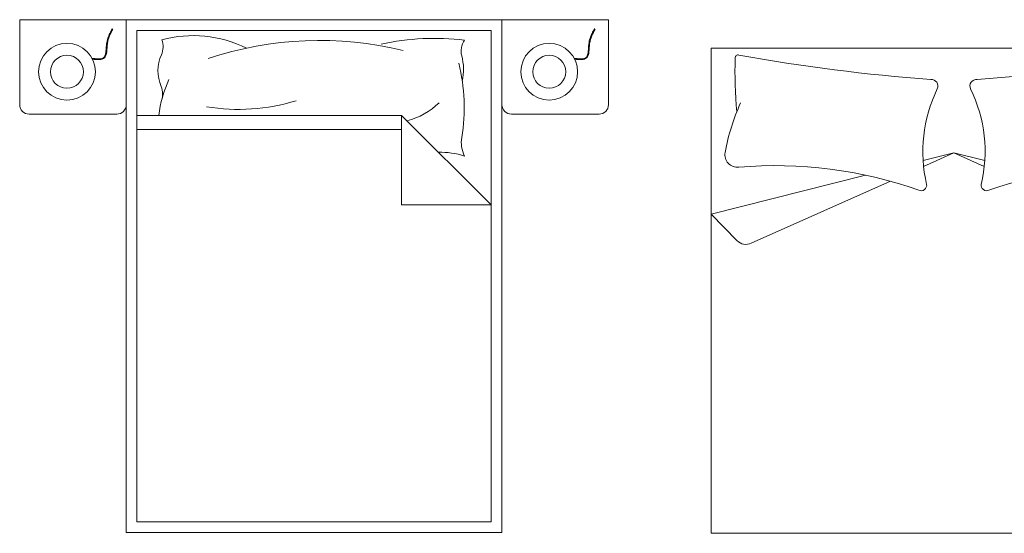
# Model space of a CAD drawing. Units: inches. Extents: x 1994 to 3075, y 3517 to 3950.
# Tile 31 of 58: x 1994.4409 to 1994.6046, y 3553.7994 to 3553.885. Entities that reach past the tile are written whole.
import ezdxf

# ---------------------------------------------------------------- set-up
doc = ezdxf.new("R2010")
doc.units = ezdxf.units.IN
doc.layers.add('A-FURN-REFR', color=8, linetype='Continuous', lineweight=13)

msp = doc.modelspace()

# ---------------------------------------------------------------- linework, layer by layer
at = {"layer": 'A-FURN-REFR'}
for p, q in [((1994.458602013046, 3553.884958485291), (1994.440885477613, 3553.884958485291)), ((1994.440885477613, 3553.884958485291), (1994.440885477613, 3553.870803096903)), ((1994.458602013046, 3553.884958485291), (1994.52109023475, 3553.884958485291)), ((1994.458602013046, 3553.799561227223), (1994.458602013046, 3553.884958485291)), ((1994.458602013046, 3553.870803096903), (1994.458602013046, 3553.884958485291)), ((1994.52109023475, 3553.799561227223), (1994.52109023475, 3553.884958485291)), ((1994.538806770183, 3553.884958485291), (1994.52109023475, 3553.884958485291)), ((1994.52109023475, 3553.884958485291), (1994.52109023475, 3553.870803096903)), ((1994.538806770183, 3553.870803096903), (1994.538806770183, 3553.884958485291)), ((1994.460391562079, 3553.801350776257), (1994.460391562079, 3553.883168936257)), ((1994.460391562079, 3553.883168936257), (1994.519300685716, 3553.883168936257)), ((1994.519300685716, 3553.883168936257), (1994.519300685716, 3553.801350776257)), ((1994.555875329129, 3553.880219755423), (1994.596260242865, 3553.880219755423)), ((1994.555875329129, 3553.880219755423), (1994.596260242865, 3553.880219755423)), ((1994.555875329129, 3553.799449927951), (1994.555875329129, 3553.880219755423)), ((1994.636645156601, 3553.880219755423), (1994.596260242865, 3553.880219755423)), ((1994.636645156601, 3553.880219755423), (1994.596260242865, 3553.880219755423)), ((1994.442460280762, 3553.869228293754), (1994.457027209896, 3553.869228293754)), ((1994.460391562079, 3553.86903075444), (1994.504377049352, 3553.86903075444)), ((1994.519300685716, 3553.854107118076), (1994.504377049352, 3553.86903075444)), ((1994.504377049352, 3553.86903075444), (1994.504377049352, 3553.854107118076)), ((1994.522665037899, 3553.869228293754), (1994.537231967033, 3553.869228293754)), ((1994.504377049352, 3553.866674390802), (1994.460391562079, 3553.866674390802)), ((1994.555875329129, 3553.799449927951), (1994.555875329129, 3553.864775123905)), ((1994.596260242865, 3553.862786175835), (1994.591129404051, 3553.861491244544)), ((1994.596260242865, 3553.862786175835), (1994.591210390106, 3553.860531295462)), ((1994.596260242865, 3553.862786175835), (1994.601391081679, 3553.861491244544)), ((1994.596260242865, 3553.862786175835), (1994.601310095624, 3553.860531295462)), ((1994.581568016439, 3553.859078122546), (1994.555864473874, 3553.852591011417)), ((1994.585689006065, 3553.858065865062), (1994.562544598623, 3553.84773133204)), ((1994.504377049352, 3553.854107118076), (1994.519300685716, 3553.854107118076)), ((1994.56016554827, 3553.848187382655), (1994.555875329129, 3553.852593751088)), ((1994.519300685716, 3553.801350776257), (1994.460391562079, 3553.801350776257)), ((1994.458602013046, 3553.799561227223), (1994.52109023475, 3553.799561227223)), ((1994.596260242865, 3553.799449927951), (1994.555875329129, 3553.799449927951)), ((1994.596260242865, 3553.799449927951), (1994.555875329129, 3553.799449927951)), ((1994.596260242865, 3553.799449927951), (1994.636645156601, 3553.799449927951)), ((1994.596260242865, 3553.799449927951), (1994.636645156601, 3553.799449927951))]:
    msp.add_line(p, q, dxfattribs=at)
for centre, radius in [((1994.448745440411, 3553.876285755194), 0.004728775123852), ((1994.448745440411, 3553.876285755194), 0.004728775123852), ((1994.528950197548, 3553.876285755194), 0.004728775123852), ((1994.528950197548, 3553.876285755194), 0.004728775123852), ((1994.448745440411, 3553.876285755194), 0.0027401859108547), ((1994.448745440411, 3553.876285755194), 0.0027401859108547), ((1994.528950197548, 3553.876285755194), 0.0027401859108547), ((1994.528950197548, 3553.876285755194), 0.0027401859108547)]:
    msp.add_circle(centre, radius, dxfattribs=at)
for centre, radius, start, end in [((1994.461538322307, 3553.880419990025), 0.0032028341489732, 335.7877323280015, 21.71237864400314), ((1994.469744612999, 3553.862561472841), 0.0197486987265365, 63.38196750841395, 105.3587807882128), ((1994.490802944634, 3553.822830045695), 0.0586716085832465, 76.33335198625635, 108.4694926903225), ((1994.509917795668, 3553.840377786862), 0.0414680575843914, 83.14136388124066, 102.4247502365447), ((1994.51739596558, 3553.879739200475), 0.0031075126812102, 144.3787648229011, 195.1987658355305), ((1994.470457361732, 3553.876409319178), 0.0065764677133891, 155.7877323280015, 202.8808293159797), ((1994.484961945259, 3553.870356990338), 0.0298558147000044, 350.3711224665587, 14.25995084780135), ((1994.506101547708, 3553.876670836297), 0.0085962787467616, 347.311957921453, 15.19876583553051), ((1994.628779041679, 3553.876029527558), 0.0689357559366832, 177.8833686819633, 185.3330513938759), ((1994.560332011409, 3553.87865222054), 0.0004482907065646, 70.44410133489674, 189.842981094497), ((1994.614290495136, 3554.173819251654), 0.2996159645214513, 259.654043260426, 265.8105338603514), ((1994.578229990593, 3554.173819251654), 0.2996159645214513, 274.1894661393186, 280.345956739574), ((1994.483724503536, 3553.86664608954), 0.0198519972069101, 155.1179531461462, 173.1008468379609), ((1994.592498233703, 3553.873909563803), 0.0010985341214448, 334.0063374253624, 95.02047578612859), ((1994.600022252026, 3553.873909563803), 0.0010985341214448, 84.97952421387143, 205.9936625746376), ((1994.461320993443, 3553.872553568025), 0.0033401870886801, 339.0160855821216, 22.88082931597971), ((1994.614853319403, 3553.863009320701), 0.0237724360313189, 154.0063374253624, 193.3195713203381), ((1994.577667166327, 3553.863009320701), 0.0237724360313189, 346.680428679662, 25.99366257463764), ((1994.477295865929, 3553.902246708011), 0.0322267158934928, 260.4320326468418, 287.2701993260345), ((1994.502530272583, 3553.879237770527), 0.0114567055564695, 283.9361364524131, 315.0098308273483), ((1994.592881340778, 3553.856579485091), 0.0352435291682938, 155.6022979544526, 169.7117845603733), ((1994.442460280762, 3553.870803096903), 0.0015748031496063, 180, 270), ((1994.457027209896, 3553.870803096903), 0.0015748031496063, 270, 0), ((1994.522665037899, 3553.870803096903), 0.0015748031496063, 180, 270), ((1994.537231967033, 3553.870803096903), 0.0015748031496063, 270, 0), ((1994.519322849789, 3553.864527463233), 0.004996088352876, 170.3711224665586, 206.9649370961853), ((1994.510759446875, 3553.849335678653), 0.0135641447689492, 72.35976010254194, 91.05260058094025), ((1994.560286636625, 3553.862496021546), 0.0021161969121165, 169.7117845603733, 274.9876097517407), ((1994.566658362432, 3553.789485019043), 0.0711723108928985, 70.4847636335054, 94.98760975174076), ((1994.625862123298, 3553.789485019043), 0.0711723108928985, 85.01239024825922, 109.5152363667157), ((1994.590818977297, 3553.857395203452), 0.0009117868872928, 245.0255496401715, 8.665342121911433), ((1994.601701508433, 3553.857395203452), 0.0009117868872928, 171.3346578780885, 294.9744503598286), ((1994.561681775446, 3553.849663642972), 0.0021161969121165, 224.234818434144, 294.0619075749208)]:
    msp.add_arc(centre, radius, start, end, dxfattribs=at)
for points, knots in [([(1994.452986283618, 3553.878377778871), (1994.453779922923, 3553.878304493638), (1994.455533490929, 3553.878155905045), (1994.455239511768, 3553.881218207943), (1994.455986431287, 3553.882661084689), (1994.456383254379, 3553.883403230019)], [0, 0, 0, 0, 0.001991930159881, 0.0044204930029738, 0.0070212840219501, 0.0070212840219501, 0.0070212840219501, 0.0070212840219501]), ([(1994.452986283618, 3553.878377778871), (1994.453779922923, 3553.878304493638), (1994.455533490929, 3553.878155905045), (1994.455239511768, 3553.881218207943), (1994.455986431287, 3553.882661084689), (1994.456383254379, 3553.883403230019)], [0, 0, 0, 0, 0.001991930159881, 0.0044204930029738, 0.0070212840219501, 0.0070212840219501, 0.0070212840219501, 0.0070212840219501]), ([(1994.452997935196, 3553.878503959135), (1994.45312235158, 3553.878492470436), (1994.453246275267, 3553.878481030475), (1994.453611847505, 3553.878451709487), (1994.453847423518, 3553.878438937463), (1994.454233671916, 3553.87845012506), (1994.454391844995, 3553.878467649254), (1994.454673798892, 3553.878539239492), (1994.454792752182, 3553.878595408417), (1994.454956845218, 3553.878738444704), (1994.455016214094, 3553.878822544618), (1994.455113368556, 3553.879031288531), (1994.455150280247, 3553.879155310755), (1994.455234024354, 3553.879571583959), (1994.455252658311, 3553.87990570344), (1994.455286098713, 3553.880475476784), (1994.455300253017, 3553.880705747389), (1994.455368517727, 3553.881257961641), (1994.455440774967, 3553.881564521784), (1994.455627258606, 3553.882141065422), (1994.455741342199, 3553.882411994596), (1994.4559939642, 3553.882944010058), (1994.456133241174, 3553.883204390223), (1994.45627150854, 3553.883462980216)], [0, 0, 0, 0, 0.7456664768345322, 0.7456664768345322, 2.236999430503596, 2.236999430503596, 3.442388313778277, 3.442388313778277, 4.740874518937371, 4.740874518937371, 5.813128485196044, 5.813128485196044, 6.885382451454717, 6.885382451454717, 9.044396613967223, 9.044396613967223, 10.46205112301665, 10.46205112301665, 12.54798424783743, 12.54798424783743, 14.63391737265821, 14.63391737265821, 16.79785288112622, 16.79785288112622, 16.79785288112622, 16.79785288112622]), ([(1994.452997935196, 3553.878503959135), (1994.45312235158, 3553.878492470436), (1994.453246275267, 3553.878481030475), (1994.453611847505, 3553.878451709487), (1994.453847423518, 3553.878438937463), (1994.454233671916, 3553.87845012506), (1994.454391844995, 3553.878467649254), (1994.454673798892, 3553.878539239492), (1994.454792752182, 3553.878595408417), (1994.454956845218, 3553.878738444704), (1994.455016214094, 3553.878822544618), (1994.455113368556, 3553.879031288531), (1994.455150280247, 3553.879155310755), (1994.455234024354, 3553.879571583959), (1994.455252658311, 3553.87990570344), (1994.455286098713, 3553.880475476784), (1994.455300253017, 3553.880705747389), (1994.455368517727, 3553.881257961641), (1994.455440774967, 3553.881564521784), (1994.455627258606, 3553.882141065422), (1994.455741342199, 3553.882411994596), (1994.4559939642, 3553.882944010058), (1994.456133241174, 3553.883204390223), (1994.45627150854, 3553.883462980216)], [0, 0, 0, 0, 0.7456664768345322, 0.7456664768345322, 2.236999430503596, 2.236999430503596, 3.442388313778277, 3.442388313778277, 4.740874518937371, 4.740874518937371, 5.813128485196044, 5.813128485196044, 6.885382451454717, 6.885382451454717, 9.044396613967223, 9.044396613967223, 10.46205112301665, 10.46205112301665, 12.54798424783743, 12.54798424783743, 14.63391737265821, 14.63391737265821, 16.79785288112622, 16.79785288112622, 16.79785288112622, 16.79785288112622]), ([(1994.533191040754, 3553.878377778871), (1994.53398468006, 3553.878304493638), (1994.535738248067, 3553.878155905047), (1994.535444268904, 3553.881218207942), (1994.536191188424, 3553.882661084688), (1994.536588011516, 3553.883403230019)], [0, 0, 0, 0, 0.001991930159881, 0.0044204930029738, 0.0070212840220299, 0.0070212840220299, 0.0070212840220299, 0.0070212840220299]), ([(1994.533191040754, 3553.878377778871), (1994.53398468006, 3553.878304493638), (1994.535738248067, 3553.878155905047), (1994.535444268904, 3553.881218207942), (1994.536191188424, 3553.882661084688), (1994.536588011516, 3553.883403230019)], [0, 0, 0, 0, 0.001991930159881, 0.0044204930029738, 0.0070212840220299, 0.0070212840220299, 0.0070212840220299, 0.0070212840220299]), ([(1994.533202692332, 3553.878503959135), (1994.533327108717, 3553.878492470436), (1994.533451032404, 3553.878481030475), (1994.533816604641, 3553.878451709487), (1994.534052180654, 3553.878438937463), (1994.534438429052, 3553.87845012506), (1994.534596602132, 3553.878467649254), (1994.534878556029, 3553.878539239492), (1994.534997509319, 3553.878595408417), (1994.535161602354, 3553.878738444704), (1994.53522097123, 3553.878822544618), (1994.535318125693, 3553.879031288531), (1994.535355037384, 3553.879155310755), (1994.53543878149, 3553.879571583959), (1994.535457415447, 3553.87990570344), (1994.53549085585, 3553.880475476784), (1994.535505010153, 3553.880705747389), (1994.535573274864, 3553.881257961641), (1994.535645532103, 3553.881564521784), (1994.535832015743, 3553.882141065422), (1994.535946099336, 3553.882411994596), (1994.536198721336, 3553.882944010058), (1994.536337998311, 3553.883204390223), (1994.536476265677, 3553.883462980216)], [0, 0, 0, 0, 0.7456664768345322, 0.7456664768345322, 2.236999430503596, 2.236999430503596, 3.442388313778277, 3.442388313778277, 4.740874518937371, 4.740874518937371, 5.813128485196044, 5.813128485196044, 6.885382451454717, 6.885382451454717, 9.044396613967223, 9.044396613967223, 10.46205112301665, 10.46205112301665, 12.54798424783743, 12.54798424783743, 14.63391737265821, 14.63391737265821, 16.79785288112622, 16.79785288112622, 16.79785288112622, 16.79785288112622]), ([(1994.533202692332, 3553.878503959135), (1994.533327108717, 3553.878492470436), (1994.533451032404, 3553.878481030475), (1994.533816604641, 3553.878451709487), (1994.534052180654, 3553.878438937463), (1994.534438429052, 3553.87845012506), (1994.534596602132, 3553.878467649254), (1994.534878556029, 3553.878539239492), (1994.534997509319, 3553.878595408417), (1994.535161602354, 3553.878738444704), (1994.53522097123, 3553.878822544618), (1994.535318125693, 3553.879031288531), (1994.535355037384, 3553.879155310755), (1994.53543878149, 3553.879571583959), (1994.535457415447, 3553.87990570344), (1994.53549085585, 3553.880475476784), (1994.535505010153, 3553.880705747389), (1994.535573274864, 3553.881257961641), (1994.535645532103, 3553.881564521784), (1994.535832015743, 3553.882141065422), (1994.535946099336, 3553.882411994596), (1994.536198721336, 3553.882944010058), (1994.536337998311, 3553.883204390223), (1994.536476265677, 3553.883462980216)], [0, 0, 0, 0, 0.7456664768345322, 0.7456664768345322, 2.236999430503596, 2.236999430503596, 3.442388313778277, 3.442388313778277, 4.740874518937371, 4.740874518937371, 5.813128485196044, 5.813128485196044, 6.885382451454717, 6.885382451454717, 9.044396613967223, 9.044396613967223, 10.46205112301665, 10.46205112301665, 12.54798424783743, 12.54798424783743, 14.63391737265821, 14.63391737265821, 16.79785288112622, 16.79785288112622, 16.79785288112622, 16.79785288112622])]:
    msp.add_open_spline(points, degree=3, knots=knots, dxfattribs=at)

doc.saveas('drawing.dxf')
